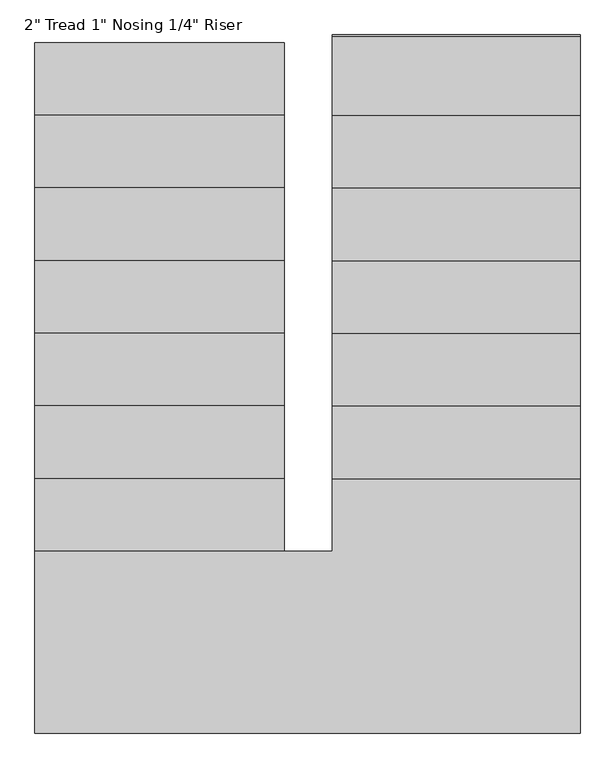
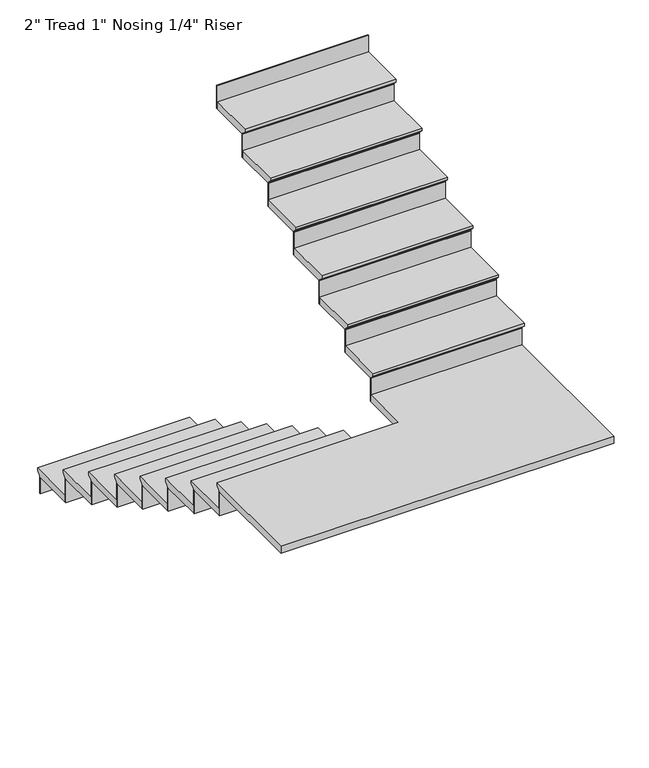
"""IFC4 building model written with IfcOpenShell, lengths in millimetres: stair flight geometry."""

from ifc_helpers import new_model, si_unit, origin, place, context, project, spatial, faceted_brep, source, transform, mapped, element, save


def stair_flight_f9143c42(model_context):
    return source(origin(), model_context, "Body", "Brep", [
        faceted_brep([(-4232.280864, -3571.6080018, 9599.0833333), (-4232.280864, -3571.6080018, 9618.1333333), (-3187.6083919, -3571.6080018, 9618.1333333), (-3187.6083919, -3571.6080018, 9599.0833333), (-4232.280864, -3597.0080018, 9573.6833333), (-3187.6083919, -3597.0080018, 9573.6833333), (-4232.280864, -3901.8080018, 9618.1333333), (-3187.6083919, -3901.8080018, 9618.1333333), (-3187.6083919, -3597.0080018, 9567.3333333), (-3187.6083919, -3901.8080018, 9567.3333333), (-4232.280864, -3901.8080018, 9567.3333333), (-4232.280864, -3597.0080018, 9567.3333333)], [[[0, 1, 2, 3]], [[4, 0, 3, 5]], [[2, 1, 6, 7]], [[8, 9, 10, 11]], [[2, 7, 9, 8, 5, 3]], [[8, 11, 4, 5]], [[6, 1, 0, 4, 11, 10]], [[7, 6, 10, 9]]]),
        faceted_brep([(-4232.280864, -3597.0080018, 9567.3333333), (-4232.280864, -3597.0080018, 9448.8), (-4232.280864, -3603.3580018, 9448.8), (-4232.280864, -3603.3580018, 9567.3333333), (-3187.6083919, -3597.0080018, 9567.3333333), (-3187.6083919, -3603.3580018, 9567.3333333), (-3187.6083919, -3603.3580018, 9448.8), (-3187.6083919, -3597.0080018, 9448.8)], [[[0, 1, 2, 3]], [[4, 5, 6, 7]], [[1, 0, 4, 7]], [[2, 1, 7, 6]], [[3, 2, 6, 5]], [[0, 3, 5, 4]]]),
        faceted_brep([(-4232.280864, -3901.8080018, 9736.6666667), (-4232.280864, -3901.8080018, 9567.3333333), (-4232.280864, -3908.1580018, 9567.3333333), (-4232.280864, -3908.1580018, 9736.6666667), (-3187.6083919, -3901.8080018, 9736.6666667), (-3187.6083919, -3908.1580018, 9736.6666667), (-3187.6083919, -3908.1580018, 9567.3333333), (-3187.6083919, -3901.8080018, 9567.3333333)], [[[0, 1, 2, 3]], [[4, 5, 6, 7]], [[1, 0, 4, 7]], [[2, 1, 7, 6]], [[3, 2, 6, 5]], [[0, 3, 5, 4]]]),
        faceted_brep([(-3187.6083919, -3876.4080018, 9787.4666667), (-4232.280864, -3876.4080018, 9787.4666667), (-4232.280864, -4206.6080018, 9787.4666667), (-3187.6083919, -4206.6080018, 9787.4666667), (-3187.6083919, -3901.8080018, 9736.6666667), (-3187.6083919, -4206.6080018, 9736.6666667), (-4232.280864, -4206.6080018, 9736.6666667), (-4232.280864, -3901.8080018, 9736.6666667), (-3187.6083919, -3901.8080018, 9743.0166667), (-3187.6083919, -3876.4080018, 9768.4166667), (-4232.280864, -3901.8080018, 9743.0166667), (-4232.280864, -3876.4080018, 9768.4166667)], [[[0, 1, 2, 3]], [[4, 5, 6, 7]], [[0, 3, 5, 4, 8, 9]], [[4, 7, 10, 8]], [[2, 1, 11, 10, 7, 6]], [[3, 2, 6, 5]], [[11, 1, 0, 9]], [[10, 11, 9, 8]]]),
        faceted_brep([(-4232.280864, -4206.6080018, 9906.0), (-4232.280864, -4206.6080018, 9736.6666667), (-4232.280864, -4212.9580018, 9736.6666667), (-4232.280864, -4212.9580018, 9906.0), (-3187.6083919, -4206.6080018, 9906.0), (-3187.6083919, -4212.9580018, 9906.0), (-3187.6083919, -4212.9580018, 9736.6666667), (-3187.6083919, -4206.6080018, 9736.6666667)], [[[0, 1, 2, 3]], [[4, 5, 6, 7]], [[1, 0, 4, 7]], [[2, 1, 7, 6]], [[3, 2, 6, 5]], [[0, 3, 5, 4]]]),
        faceted_brep([(-3187.6083919, -4181.2080018, 9956.8), (-4232.280864, -4181.2080018, 9956.8), (-4232.280864, -4511.4080018, 9956.8), (-3187.6083919, -4511.4080018, 9956.8), (-3187.6083919, -4206.6080018, 9906.0), (-3187.6083919, -4511.4080018, 9906.0), (-4232.280864, -4511.4080018, 9906.0), (-4232.280864, -4206.6080018, 9906.0), (-3187.6083919, -4206.6080018, 9912.35), (-3187.6083919, -4181.2080018, 9937.75), (-4232.280864, -4206.6080018, 9912.35), (-4232.280864, -4181.2080018, 9937.75)], [[[0, 1, 2, 3]], [[4, 5, 6, 7]], [[0, 3, 5, 4, 8, 9]], [[4, 7, 10, 8]], [[2, 1, 11, 10, 7, 6]], [[3, 2, 6, 5]], [[11, 1, 0, 9]], [[10, 11, 9, 8]]]),
        faceted_brep([(-4232.280864, -4511.4080018, 10075.3333333), (-4232.280864, -4511.4080018, 9906.0), (-4232.280864, -4517.7580018, 9906.0), (-4232.280864, -4517.7580018, 10075.3333333), (-3187.6083919, -4511.4080018, 10075.3333333), (-3187.6083919, -4517.7580018, 10075.3333333), (-3187.6083919, -4517.7580018, 9906.0), (-3187.6083919, -4511.4080018, 9906.0)], [[[0, 1, 2, 3]], [[4, 5, 6, 7]], [[1, 0, 4, 7]], [[2, 1, 7, 6]], [[3, 2, 6, 5]], [[0, 3, 5, 4]]]),
        faceted_brep([(-3187.6083919, -4486.0080018, 10126.1333333), (-4232.280864, -4486.0080018, 10126.1333333), (-4232.280864, -4816.2080018, 10126.1333333), (-3187.6083919, -4816.2080018, 10126.1333333), (-3187.6083919, -4511.4080018, 10075.3333333), (-3187.6083919, -4816.2080018, 10075.3333333), (-4232.280864, -4816.2080018, 10075.3333333), (-4232.280864, -4511.4080018, 10075.3333333), (-3187.6083919, -4511.4080018, 10081.6833333), (-3187.6083919, -4486.0080018, 10107.0833333), (-4232.280864, -4511.4080018, 10081.6833333), (-4232.280864, -4486.0080018, 10107.0833333)], [[[0, 1, 2, 3]], [[4, 5, 6, 7]], [[0, 3, 5, 4, 8, 9]], [[4, 7, 10, 8]], [[2, 1, 11, 10, 7, 6]], [[3, 2, 6, 5]], [[11, 1, 0, 9]], [[10, 11, 9, 8]]]),
        faceted_brep([(-4232.280864, -4816.2080018, 10244.6666667), (-4232.280864, -4816.2080018, 10075.3333333), (-4232.280864, -4822.5580018, 10075.3333333), (-4232.280864, -4822.5580018, 10244.6666667), (-3187.6083919, -4816.2080018, 10244.6666667), (-3187.6083919, -4822.5580018, 10244.6666667), (-3187.6083919, -4822.5580018, 10075.3333333), (-3187.6083919, -4816.2080018, 10075.3333333)], [[[0, 1, 2, 3]], [[4, 5, 6, 7]], [[1, 0, 4, 7]], [[2, 1, 7, 6]], [[3, 2, 6, 5]], [[0, 3, 5, 4]]]),
        faceted_brep([(-3187.6083919, -4790.8080018, 10295.4666667), (-4232.280864, -4790.8080018, 10295.4666667), (-4232.280864, -5121.0080018, 10295.4666667), (-3187.6083919, -5121.0080018, 10295.4666667), (-3187.6083919, -4816.2080018, 10244.6666667), (-3187.6083919, -5121.0080018, 10244.6666667), (-4232.280864, -5121.0080018, 10244.6666667), (-4232.280864, -4816.2080018, 10244.6666667), (-3187.6083919, -4816.2080018, 10251.0166667), (-3187.6083919, -4790.8080018, 10276.4166667), (-4232.280864, -4816.2080018, 10251.0166667), (-4232.280864, -4790.8080018, 10276.4166667)], [[[0, 1, 2, 3]], [[4, 5, 6, 7]], [[0, 3, 5, 4, 8, 9]], [[4, 7, 10, 8]], [[2, 1, 11, 10, 7, 6]], [[3, 2, 6, 5]], [[11, 1, 0, 9]], [[10, 11, 9, 8]]]),
        faceted_brep([(-4232.280864, -5121.0080018, 10414.0), (-4232.280864, -5121.0080018, 10244.6666667), (-4232.280864, -5127.3580018, 10244.6666667), (-4232.280864, -5127.3580018, 10414.0), (-3187.6083919, -5121.0080018, 10414.0), (-3187.6083919, -5127.3580018, 10414.0), (-3187.6083919, -5127.3580018, 10244.6666667), (-3187.6083919, -5121.0080018, 10244.6666667)], [[[0, 1, 2, 3]], [[4, 5, 6, 7]], [[1, 0, 4, 7]], [[2, 1, 7, 6]], [[3, 2, 6, 5]], [[0, 3, 5, 4]]]),
        faceted_brep([(-3187.6083919, -5095.6080018, 10464.8), (-4232.280864, -5095.6080018, 10464.8), (-4232.280864, -5425.8080018, 10464.8), (-3187.6083919, -5425.8080018, 10464.8), (-3187.6083919, -5121.0080018, 10414.0), (-3187.6083919, -5425.8080018, 10414.0), (-4232.280864, -5425.8080018, 10414.0), (-4232.280864, -5121.0080018, 10414.0), (-3187.6083919, -5121.0080018, 10420.35), (-3187.6083919, -5095.6080018, 10445.75), (-4232.280864, -5121.0080018, 10420.35), (-4232.280864, -5095.6080018, 10445.75)], [[[0, 1, 2, 3]], [[4, 5, 6, 7]], [[0, 3, 5, 4, 8, 9]], [[4, 7, 10, 8]], [[2, 1, 11, 10, 7, 6]], [[3, 2, 6, 5]], [[11, 1, 0, 9]], [[10, 11, 9, 8]]]),
        faceted_brep([(-4232.280864, -5425.8080018, 10583.3333333), (-4232.280864, -5425.8080018, 10414.0), (-4232.280864, -5432.1580018, 10414.0), (-4232.280864, -5432.1580018, 10583.3333333), (-3187.6083919, -5425.8080018, 10583.3333333), (-3187.6083919, -5432.1580018, 10583.3333333), (-3187.6083919, -5432.1580018, 10414.0), (-3187.6083919, -5425.8080018, 10414.0)], [[[0, 1, 2, 3]], [[4, 5, 6, 7]], [[1, 0, 4, 7]], [[2, 1, 7, 6]], [[3, 2, 6, 5]], [[0, 3, 5, 4]]]),
        faceted_brep([(-3187.6083919, -5400.4080018, 10634.1333333), (-4232.280864, -5400.4080018, 10634.1333333), (-4232.280864, -5730.6080018, 10634.1333333), (-3187.6083919, -5730.6080018, 10634.1333333), (-3187.6083919, -5425.8080018, 10583.3333333), (-3187.6083919, -5730.6080018, 10583.3333333), (-4232.280864, -5730.6080018, 10583.3333333), (-4232.280864, -5425.8080018, 10583.3333333), (-3187.6083919, -5425.8080018, 10589.6833333), (-3187.6083919, -5400.4080018, 10615.0833333), (-4232.280864, -5425.8080018, 10589.6833333), (-4232.280864, -5400.4080018, 10615.0833333)], [[[0, 1, 2, 3]], [[4, 5, 6, 7]], [[0, 3, 5, 4, 8, 9]], [[4, 7, 10, 8]], [[2, 1, 11, 10, 7, 6]], [[3, 2, 6, 5]], [[11, 1, 0, 9]], [[10, 11, 9, 8]]]),
        faceted_brep([(-4232.280864, -5730.6080018, 10752.6666667), (-4232.280864, -5730.6080018, 10583.3333333), (-4232.280864, -5736.9580018, 10583.3333333), (-4232.280864, -5736.9580018, 10752.6666667), (-3187.6083919, -5730.6080018, 10752.6666667), (-3187.6083919, -5736.9580018, 10752.6666667), (-3187.6083919, -5736.9580018, 10583.3333333), (-3187.6083919, -5730.6080018, 10583.3333333)], [[[0, 1, 2, 3]], [[4, 5, 6, 7]], [[1, 0, 4, 7]], [[2, 1, 7, 6]], [[3, 2, 6, 5]], [[0, 3, 5, 4]]]),
        faceted_brep([(-2984.4083919, -5375.0080018, 10803.4666667), (-2984.4083919, -5705.2080018, 10803.4666667), (-4232.280864, -5705.2080018, 10803.4666667), (-4232.280864, -6467.2080018, 10803.4666667), (-1946.280864, -6467.2080018, 10803.4666667), (-1946.280864, -5375.0080018, 10803.4666667), (-2984.4083919, -5705.2080018, 10752.6666667), (-2984.4083919, -5375.0080018, 10752.6666667), (-1946.280864, -5375.0080018, 10752.6666667), (-1946.280864, -6467.2080018, 10752.6666667), (-4232.280864, -6467.2080018, 10752.6666667), (-4232.280864, -5730.6080018, 10752.6666667), (-3187.6083919, -5730.6080018, 10752.6666667), (-3187.6083919, -5705.2080018, 10752.6666667), (-3187.6083919, -5705.2080018, 10784.4166667), (-4232.280864, -5705.2080018, 10784.4166667), (-3187.6083919, -5730.6080018, 10759.0166667), (-4232.280864, -5730.6080018, 10759.0166667)], [[[0, 1, 2, 3, 4, 5]], [[6, 7, 8, 9, 10, 11, 12, 13]], [[1, 0, 7, 6]], [[2, 1, 6, 13, 14, 15]], [[13, 12, 16, 14]], [[12, 11, 17, 16]], [[3, 2, 15, 17, 11, 10]], [[4, 3, 10, 9]], [[5, 4, 9, 8]], [[0, 5, 8, 7]], [[17, 15, 14, 16]]]),
        faceted_brep([(-1946.280864, -5375.0080018, 10922.0), (-1946.280864, -5375.0080018, 10752.6666667), (-1946.280864, -5368.6580018, 10752.6666667), (-1946.280864, -5368.6580018, 10922.0), (-2984.4083919, -5375.0080018, 10922.0), (-2984.4083919, -5368.6580018, 10922.0), (-2984.4083919, -5368.6580018, 10752.6666667), (-2984.4083919, -5375.0080018, 10752.6666667)], [[[0, 1, 2, 3]], [[4, 5, 6, 7]], [[1, 0, 4, 7]], [[2, 1, 7, 6]], [[3, 2, 6, 5]], [[0, 3, 5, 4]]]),
        faceted_brep([(-2984.4083919, -5400.4080018, 10972.8), (-1946.280864, -5400.4080018, 10972.8), (-1946.280864, -5070.2080018, 10972.8), (-2984.4083919, -5070.2080018, 10972.8), (-2984.4083919, -5375.0080018, 10922.0), (-2984.4083919, -5070.2080018, 10922.0), (-1946.280864, -5070.2080018, 10922.0), (-1946.280864, -5375.0080018, 10922.0), (-2984.4083919, -5375.0080018, 10928.35), (-2984.4083919, -5400.4080018, 10953.75), (-1946.280864, -5375.0080018, 10928.35), (-1946.280864, -5400.4080018, 10953.75)], [[[0, 1, 2, 3]], [[4, 5, 6, 7]], [[0, 3, 5, 4, 8, 9]], [[4, 7, 10, 8]], [[2, 1, 11, 10, 7, 6]], [[3, 2, 6, 5]], [[11, 1, 0, 9]], [[10, 11, 9, 8]]]),
        faceted_brep([(-1946.280864, -5070.2080018, 11091.3333333), (-1946.280864, -5070.2080018, 10922.0), (-1946.280864, -5063.8580018, 10922.0), (-1946.280864, -5063.8580018, 11091.3333333), (-2984.4083919, -5070.2080018, 11091.3333333), (-2984.4083919, -5063.8580018, 11091.3333333), (-2984.4083919, -5063.8580018, 10922.0), (-2984.4083919, -5070.2080018, 10922.0)], [[[0, 1, 2, 3]], [[4, 5, 6, 7]], [[1, 0, 4, 7]], [[2, 1, 7, 6]], [[3, 2, 6, 5]], [[0, 3, 5, 4]]]),
        faceted_brep([(-2984.4083919, -5095.6080018, 11142.1333333), (-1946.280864, -5095.6080018, 11142.1333333), (-1946.280864, -4765.4080018, 11142.1333333), (-2984.4083919, -4765.4080018, 11142.1333333), (-2984.4083919, -5070.2080018, 11091.3333333), (-2984.4083919, -4765.4080018, 11091.3333333), (-1946.280864, -4765.4080018, 11091.3333333), (-1946.280864, -5070.2080018, 11091.3333333), (-2984.4083919, -5070.2080018, 11097.6833333), (-2984.4083919, -5095.6080018, 11123.0833333), (-1946.280864, -5070.2080018, 11097.6833333), (-1946.280864, -5095.6080018, 11123.0833333)], [[[0, 1, 2, 3]], [[4, 5, 6, 7]], [[0, 3, 5, 4, 8, 9]], [[4, 7, 10, 8]], [[2, 1, 11, 10, 7, 6]], [[3, 2, 6, 5]], [[11, 1, 0, 9]], [[10, 11, 9, 8]]]),
        faceted_brep([(-1946.280864, -4765.4080018, 11260.6666667), (-1946.280864, -4765.4080018, 11091.3333333), (-1946.280864, -4759.0580018, 11091.3333333), (-1946.280864, -4759.0580018, 11260.6666667), (-2984.4083919, -4765.4080018, 11260.6666667), (-2984.4083919, -4759.0580018, 11260.6666667), (-2984.4083919, -4759.0580018, 11091.3333333), (-2984.4083919, -4765.4080018, 11091.3333333)], [[[0, 1, 2, 3]], [[4, 5, 6, 7]], [[1, 0, 4, 7]], [[2, 1, 7, 6]], [[3, 2, 6, 5]], [[0, 3, 5, 4]]]),
        faceted_brep([(-2984.4083919, -4790.8080018, 11311.4666667), (-1946.280864, -4790.8080018, 11311.4666667), (-1946.280864, -4460.6080018, 11311.4666667), (-2984.4083919, -4460.6080018, 11311.4666667), (-2984.4083919, -4765.4080018, 11260.6666667), (-2984.4083919, -4460.6080018, 11260.6666667), (-1946.280864, -4460.6080018, 11260.6666667), (-1946.280864, -4765.4080018, 11260.6666667), (-2984.4083919, -4765.4080018, 11267.0166667), (-2984.4083919, -4790.8080018, 11292.4166667), (-1946.280864, -4765.4080018, 11267.0166667), (-1946.280864, -4790.8080018, 11292.4166667)], [[[0, 1, 2, 3]], [[4, 5, 6, 7]], [[0, 3, 5, 4, 8, 9]], [[4, 7, 10, 8]], [[2, 1, 11, 10, 7, 6]], [[3, 2, 6, 5]], [[11, 1, 0, 9]], [[10, 11, 9, 8]]]),
        faceted_brep([(-1946.280864, -4460.6080018, 11430.0), (-1946.280864, -4460.6080018, 11260.6666667), (-1946.280864, -4454.2580018, 11260.6666667), (-1946.280864, -4454.2580018, 11430.0), (-2984.4083919, -4460.6080018, 11430.0), (-2984.4083919, -4454.2580018, 11430.0), (-2984.4083919, -4454.2580018, 11260.6666667), (-2984.4083919, -4460.6080018, 11260.6666667)], [[[0, 1, 2, 3]], [[4, 5, 6, 7]], [[1, 0, 4, 7]], [[2, 1, 7, 6]], [[3, 2, 6, 5]], [[0, 3, 5, 4]]]),
        faceted_brep([(-2984.4083919, -4486.0080018, 11480.8), (-1946.280864, -4486.0080018, 11480.8), (-1946.280864, -4155.8080018, 11480.8), (-2984.4083919, -4155.8080018, 11480.8), (-2984.4083919, -4460.6080018, 11430.0), (-2984.4083919, -4155.8080018, 11430.0), (-1946.280864, -4155.8080018, 11430.0), (-1946.280864, -4460.6080018, 11430.0), (-2984.4083919, -4460.6080018, 11436.35), (-2984.4083919, -4486.0080018, 11461.75), (-1946.280864, -4460.6080018, 11436.35), (-1946.280864, -4486.0080018, 11461.75)], [[[0, 1, 2, 3]], [[4, 5, 6, 7]], [[0, 3, 5, 4, 8, 9]], [[4, 7, 10, 8]], [[2, 1, 11, 10, 7, 6]], [[3, 2, 6, 5]], [[11, 1, 0, 9]], [[10, 11, 9, 8]]]),
        faceted_brep([(-1946.280864, -4155.8080018, 11599.3333333), (-1946.280864, -4155.8080018, 11430.0), (-1946.280864, -4149.4580018, 11430.0), (-1946.280864, -4149.4580018, 11599.3333333), (-2984.4083919, -4155.8080018, 11599.3333333), (-2984.4083919, -4149.4580018, 11599.3333333), (-2984.4083919, -4149.4580018, 11430.0), (-2984.4083919, -4155.8080018, 11430.0)], [[[0, 1, 2, 3]], [[4, 5, 6, 7]], [[1, 0, 4, 7]], [[2, 1, 7, 6]], [[3, 2, 6, 5]], [[0, 3, 5, 4]]]),
        faceted_brep([(-2984.4083919, -4181.2080018, 11650.1333333), (-1946.280864, -4181.2080018, 11650.1333333), (-1946.280864, -3851.0080018, 11650.1333333), (-2984.4083919, -3851.0080018, 11650.1333333), (-2984.4083919, -4155.8080018, 11599.3333333), (-2984.4083919, -3851.0080018, 11599.3333333), (-1946.280864, -3851.0080018, 11599.3333333), (-1946.280864, -4155.8080018, 11599.3333333), (-2984.4083919, -4155.8080018, 11605.6833333), (-2984.4083919, -4181.2080018, 11631.0833333), (-1946.280864, -4155.8080018, 11605.6833333), (-1946.280864, -4181.2080018, 11631.0833333)], [[[0, 1, 2, 3]], [[4, 5, 6, 7]], [[0, 3, 5, 4, 8, 9]], [[4, 7, 10, 8]], [[2, 1, 11, 10, 7, 6]], [[3, 2, 6, 5]], [[11, 1, 0, 9]], [[10, 11, 9, 8]]]),
        faceted_brep([(-1946.280864, -3851.0080018, 11768.6666667), (-1946.280864, -3851.0080018, 11599.3333333), (-1946.280864, -3844.6580018, 11599.3333333), (-1946.280864, -3844.6580018, 11768.6666667), (-2984.4083919, -3851.0080018, 11768.6666667), (-2984.4083919, -3844.6580018, 11768.6666667), (-2984.4083919, -3844.6580018, 11599.3333333), (-2984.4083919, -3851.0080018, 11599.3333333)], [[[0, 1, 2, 3]], [[4, 5, 6, 7]], [[1, 0, 4, 7]], [[2, 1, 7, 6]], [[3, 2, 6, 5]], [[0, 3, 5, 4]]]),
        faceted_brep([(-1946.280864, -3546.2080018, 11938.0), (-1946.280864, -3546.2080018, 11768.6666667), (-1946.280864, -3539.8580018, 11768.6666667), (-1946.280864, -3539.8580018, 11938.0), (-2984.4083919, -3546.2080018, 11938.0), (-2984.4083919, -3539.8580018, 11938.0), (-2984.4083919, -3539.8580018, 11768.6666667), (-2984.4083919, -3546.2080018, 11768.6666667)], [[[0, 1, 2, 3]], [[4, 5, 6, 7]], [[1, 0, 4, 7]], [[2, 1, 7, 6]], [[3, 2, 6, 5]], [[0, 3, 5, 4]]]),
        faceted_brep([(-2984.4083919, -3876.4080018, 11819.4666667), (-1946.280864, -3876.4080018, 11819.4666667), (-1946.280864, -3546.2080018, 11819.4666667), (-2984.4083919, -3546.2080018, 11819.4666667), (-2984.4083919, -3851.0080018, 11768.6666667), (-2984.4083919, -3546.2080018, 11768.6666667), (-1946.280864, -3546.2080018, 11768.6666667), (-1946.280864, -3851.0080018, 11768.6666667), (-2984.4083919, -3851.0080018, 11775.0166667), (-2984.4083919, -3876.4080018, 11800.4166667), (-1946.280864, -3851.0080018, 11775.0166667), (-1946.280864, -3876.4080018, 11800.4166667)], [[[0, 1, 2, 3]], [[4, 5, 6, 7]], [[0, 3, 5, 4, 8, 9]], [[4, 7, 10, 8]], [[2, 1, 11, 10, 7, 6]], [[3, 2, 6, 5]], [[11, 1, 0, 9]], [[10, 11, 9, 8]]]),
    ])


if __name__ == "__main__":
    model = new_model("IFC4")
    model_context = context("Model", 3, world=origin())
    ifc_project = project(units=[si_unit("LENGTHUNIT", "METRE", prefix="MILLI")], contexts=[model_context])
    site = spatial("IfcSite", under=ifc_project)
    building = spatial("IfcBuilding", under=site)
    placement = place(None, origin())
    stair_flight_shape = stair_flight_f9143c42(model_context)
    element("IfcStairFlight", 1, ObjectType="2\" Tread 1\" Nosing 1/4\" Riser", at=placement, inside=building, context=model_context, shape_type="MappedRepresentation", body=[
        mapped(stair_flight_shape, transform((0.0, 0.0, 0.0), x_axis=(1.0, 0.0, 0.0), y_axis=(0.0, 1.0, 0.0), z_axis=(0.0, 0.0, 1.0))),
    ])
    save(model, "model.ifc")
